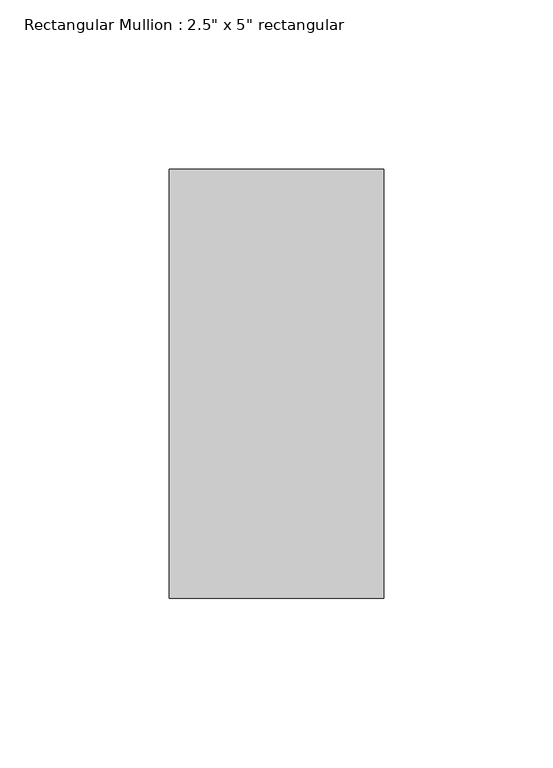
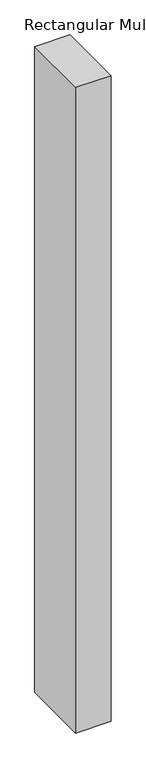
"""IFC4 building model written with IfcOpenShell, lengths in millimetres: member geometry."""

from ifc_helpers import new_model, si_unit, frame, origin, place, context, project, spatial, polyline, outline, extrude, source, transform, mapped, element, save


def member_05917e3b(model_context):
    return source(origin(), model_context, "Body", "SweptSolid", [
        extrude(outline(polyline([(0.0, 63.5), (0.0, -63.5), (-63.5, -63.5), (-63.5, 63.5), (0.0, 63.5)])), frame((0.0, 0.0, -1222.7823245), z_axis=(0.0, 0.0, 1.0), x_axis=(1.0, 0.0, 0.0)), (0.0, 0.0, 1.0), 1222.7823245),
    ])


if __name__ == "__main__":
    model = new_model("IFC4")
    model_context = context("Model", 3, world=origin())
    ifc_project = project(units=[si_unit("LENGTHUNIT", "METRE", prefix="MILLI")], contexts=[model_context])
    site = spatial("IfcSite", under=ifc_project)
    building = spatial("IfcBuilding", under=site)
    placement = place(None, origin())
    member_shape = member_05917e3b(model_context)
    element("IfcMember", 1, ObjectType="Rectangular Mullion : 2.5\" x 5\" rectangular", at=placement, inside=building, context=model_context, shape_type="MappedRepresentation", body=[
        mapped(member_shape, transform((0.0, 0.0, 0.0), x_axis=(1.0, 0.0, 0.0), y_axis=(0.0, 1.0, 0.0), z_axis=(0.0, 0.0, 1.0))),
    ])
    save(model, "model.ifc")

# Revit data of these elements
# Type "Rectangular Mullion : 2.5\" x 5\" rectangular"
#   built-in parameter 1007304 = 0.416667 (stored number, unit not read)
#   built-in parameter 1007301 = 0.104167 (stored number, unit not read)
#   built-in parameter 1007300 = 0.104167 (stored number, unit not read)
# Element 1 (IfcMember, "Rectangular Mullion : 2.5\" x 5\" rectangular")
#   Materials on its faces: "Aluminum"
# Materials
#   "Aluminum": class "Metal", colour RGB 247 247 247, transparency 0, Description = "Aluminum 6061", Cost = 0
